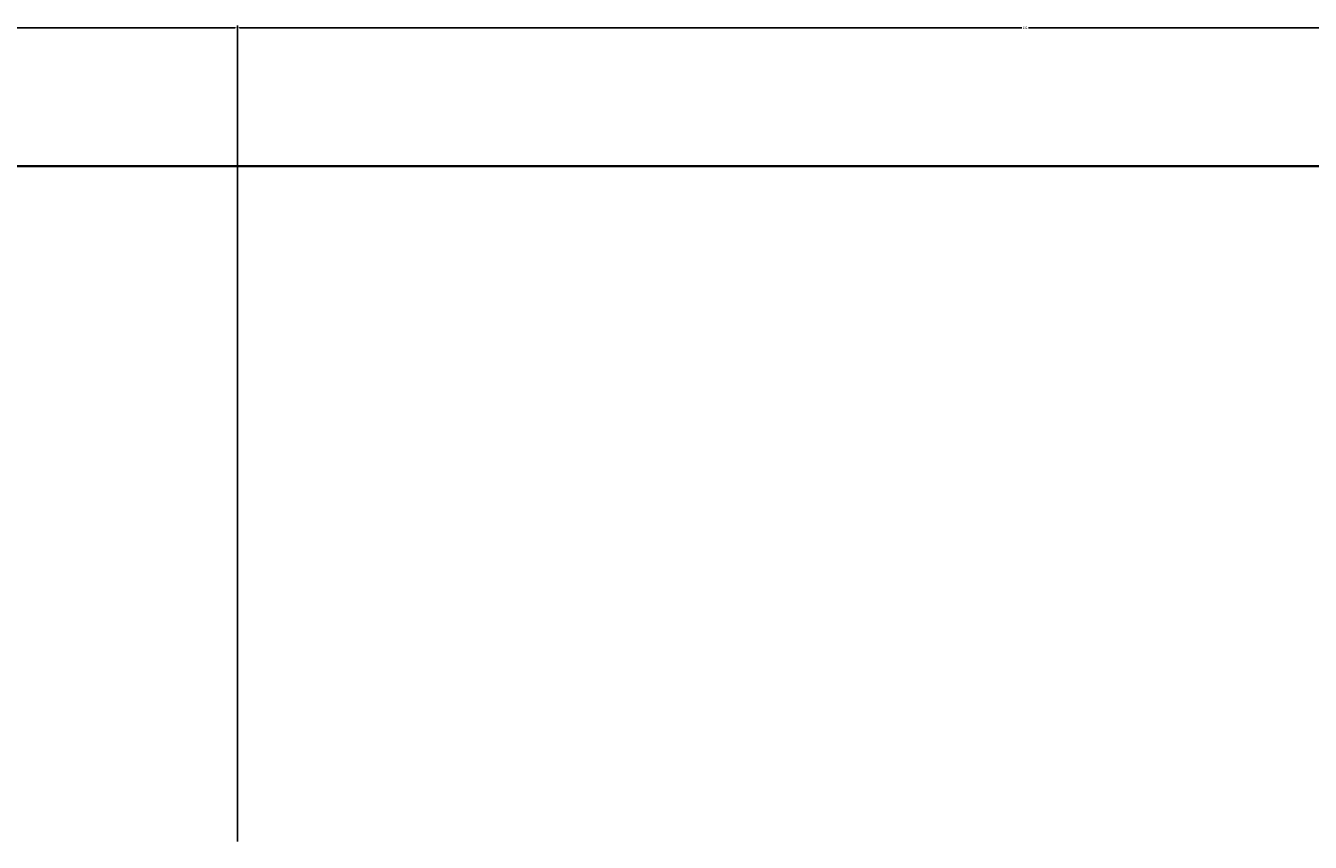
# Model space of a CAD drawing. Units: inches. Extents: x 1885 to 2748, y 783 to 2421.
# Tile 100 of 117: x 2341 to 2449, y 2353 to 2421. Entities that reach past the tile are written whole.
import ezdxf

# ---------------------------------------------------------------- set-up
doc = ezdxf.new("R2010")
doc.units = ezdxf.units.IN
doc.layers.add('A-ANNO-DIMS', color=2, linetype='Continuous', lineweight=18)
doc.layers.add('A-ANNO-TTLB', color=7, linetype='Continuous', lineweight=35)
doc.styles.get("Standard").update_dxf_attribs({"font": 'arial.ttf'})
doc.dimstyles.get("Standard").update_dxf_attribs({"dimtxt": 0.18, "dimasz": 0.18, "dimexe": 0.18, "dimexo": 0.0625, "dimgap": 0.09, "dimtad": 0, "dimtih": 1, "dimtoh": 1, "dimdec": 4, "dimzin": 0, "dimdsep": 46, "dimtxsty": 'Standard', "dimcen": 0.09, "dimadec": 0, "dimazin": 0, "dimtfac": 1, "dimtdec": 4, "dimtofl": 0, "dimtmove": 0, "dimatfit": 3, "dimfxl": 1, "dimtolj": 1, "dimtzin": 0, "dimarcsym": 0})

# ---------------------------------------------------------------- blocks, each defined once
blk = doc.blocks.new('*D52')
at = {"layer": 'A-ANNO-DIMS', "color": 0, "lineweight": -2, "transparency": 16777216}
for p, q in [((2310.77, 2348.07), (2310.77, 2420.94)), ((2310.95, 2420.76), (2334.55, 2420.76)), ((2358.59, 2420.76), (2335, 2420.76)), ((2358.77, 2352.57), (2358.77, 2420.94))]:
    blk.add_line(p, q, dxfattribs=at)
at = {"layer": 'A-ANNO-DIMS', "color": 0, "transparency": 16777216}
for points in [[(2310.95, 2420.79), (2310.95, 2420.73), (2310.77, 2420.76)], [(2358.59, 2420.79), (2358.59, 2420.73), (2358.77, 2420.76)]]:
    blk.add_solid(points, dxfattribs=at)
at = {"layer": 'Defpoints', "color": 0, "transparency": 16777216}
for p in [(2358.77, 2420.76), (2358.77, 2352.51), (2310.77, 2348.01)]:
    blk.add_point(p, dxfattribs=at)
at = {"layer": 'A-ANNO-DIMS', "color": 0, "transparency": 16777216, "insert": (2334.77, 2420.76), "char_height": 0.18, "attachment_point": 5}
blk.add_mtext('\\A1;48', dxfattribs=at)
blk = doc.blocks.new('*D53')
at = {"layer": 'A-ANNO-DIMS', "color": 0, "lineweight": -2, "transparency": 16777216}
for p, q in [((2358.77, 2352.57), (2358.77, 2420.94)), ((2358.95, 2420.76), (2424.49, 2420.76)), ((2490.59, 2420.76), (2425.05, 2420.76)), ((2490.77, 2352.57), (2490.77, 2420.94))]:
    blk.add_line(p, q, dxfattribs=at)
at = {"layer": 'A-ANNO-DIMS', "color": 0, "transparency": 16777216}
for points in [[(2358.95, 2420.79), (2358.95, 2420.73), (2358.77, 2420.76)], [(2490.59, 2420.79), (2490.59, 2420.73), (2490.77, 2420.76)]]:
    blk.add_solid(points, dxfattribs=at)
at = {"layer": 'Defpoints', "color": 0, "transparency": 16777216}
for p in [(2490.77, 2420.76), (2358.77, 2352.51), (2490.77, 2352.51)]:
    blk.add_point(p, dxfattribs=at)
at = {"layer": 'A-ANNO-DIMS', "color": 0, "transparency": 16777216, "insert": (2424.77, 2420.76), "char_height": 0.18, "attachment_point": 5}
blk.add_mtext('\\A1;132', dxfattribs=at)

msp = doc.modelspace()

# ---------------------------------------------------------------- linework, layer by layer
at = {"layer": 'A-ANNO-TTLB'}
msp.add_lwpolyline([(1885.16, 2409.17), (2748.2, 2409.17), (2748.2, 922.58), (1885.16, 922.58)], close=True, dxfattribs=at)

# ---------------------------------------------------------------- dimensions: what is measured, and where the dimension line sits
at = {"layer": 'A-ANNO-DIMS'}
for base, p1, p2, picture, middle in [((2358.77, 2420.76), (2310.77, 2348.01), (2358.77, 2352.51), '*D52', (2334.77, 2420.76)), ((2490.77, 2420.76), (2358.77, 2352.51), (2490.77, 2352.51), '*D53', (2424.77, 2420.76))]:
    dim = msp.add_linear_dim(base=base, p1=p1, p2=p2, dimstyle='Standard', override={"dimdec": 0, "dimlfac": 1, "dimrnd": 0, "dimzin": 0, "dimdsep": 46, "dimlunit": 2}, dxfattribs=at)
    dim.commit()
    dim.dimension.update_dxf_attribs({"geometry": picture, "text_midpoint": middle})

doc.saveas('drawing.dxf')
